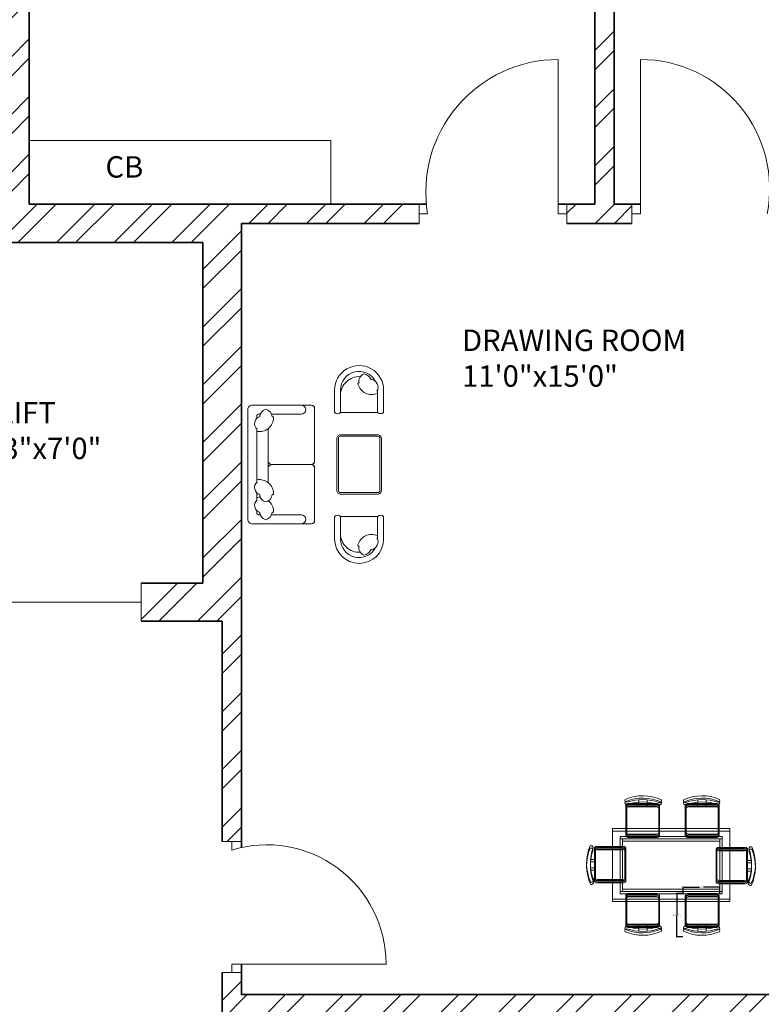
# Model space of a CAD drawing. Units: inches. Extents: x 2168 to 3056, y 1130 to 2629.
# Tile 33 of 42: x 2598 to 2771, y 2079 to 2308. Entities that reach past the tile are written whole.
import ezdxf

# ---------------------------------------------------------------- set-up
doc = ezdxf.new("R2010")
doc.units = ezdxf.units.IN
for name, color, linetype, lineweight in [('A-ANNO-DIMS', 2, 'Continuous', 18), ('A-ANNO-TEXT', 7, 'Continuous', 18), ('A-AREA-IDEN', 7, 'Continuous', 18), ('A-DOOR', 21, 'Continuous', 18), ('A-EQPM-ELEV', 7, 'Continuous', 18), ('A-FLOR-CASE', 71, 'Continuous', 18), ('A-FURN', 8, 'Continuous', 13), ('A-WALL', 7, 'Continuous', 35)]:
    doc.layers.add(name, color=color, linetype=linetype, lineweight=lineweight)
doc.layers.add('A-WALL-PATT', color=143, linetype='Continuous', lineweight=13, true_color=0x7aafdf)
doc.styles.get("Standard").update_dxf_attribs({"font": 'arial.ttf'})
doc.dimstyles.get("Standard").update_dxf_attribs({"dimtxt": 0.18, "dimasz": 0.18, "dimexe": 0.18, "dimexo": 0.0625, "dimgap": 0.09, "dimtad": 0, "dimtih": 1, "dimtoh": 1, "dimdec": 4, "dimzin": 0, "dimdsep": 46, "dimtxsty": 'Standard', "dimcen": 0.09, "dimadec": 0, "dimazin": 0, "dimtfac": 1, "dimtdec": 4, "dimtofl": 0, "dimtmove": 0, "dimatfit": 3, "dimfxl": 1, "dimtolj": 1, "dimtzin": 0, "dimarcsym": 0})

# ---------------------------------------------------------------- blocks, each defined once
blk = doc.blocks.new('A$C1352')
at = {"color": 0}
for points in [[(0.003, 0.053), (0.003, 0.553, -0.414214), (0.053, 0.603), (0.753, 0.603, -0.414214), (0.803, 0.553), (0.803, 0.053, -0.414214), (0.753, 0.003), (0.053, 0.003, -0.414214)], [(0.023, 0.053), (0.023, 0.553, -0.414214), (0.053, 0.583), (0.753, 0.583, -0.414214), (0.783, 0.553), (0.783, 0.053, -0.414214), (0.753, 0.023), (0.053, 0.023, -0.414214)]]:
    blk.add_lwpolyline(points, format="xyb", close=True, dxfattribs=at)
blk = doc.blocks.new('CHAIR-LOUNGE')
blk.add_line((10.04, 5.71), (10.04, 10.98))
at = {"ltscale": 0.03}
blk.add_lwpolyline([(10.04, 10.98, -0.369229), (11.42, 10.98), (11.42, 5.7, -1), (0, 5.72), (0, 10.99, -0.369229), (1.39, 10.99)], format="xyb", close=True, dxfattribs=at)
blk.add_lwpolyline([(9.55, 3.71, -0.785087), (1.38, 5.71), (1.39, 10.99)], format="xyb")
for centre, radius, start, end in [((5.71, 6.93), 4.33, 179.9461, 273.658), ((8.67, 3.43), 3.35, 67.0143, 164.2857), ((8.41, 5.02), 1.73, 272.9922, 34.1401), ((5.71, 5.71), 4.33, 358.8536, 359.9461), ((5.63, 4.23), 0.207, 150.6238, 293.7423), ((7.44, 3.63), 1.78, 166.6403, 249.4695), ((6.65, 3.91), 1.95, 274.9999, 341.3534)]:
    blk.add_arc(centre, radius, start, end)
blk = doc.blocks.new('TABLE-DINING')
for points in [[(0, 17.02), (27.45, 17.02), (27.45, 0.55), (0, 0.55)], [(0, 17.02), (27.45, 17.02), (27.45, 0.55), (0, 0.55)], [(0, 16.47), (27.45, 16.47), (27.45, 0), (0, 0)], [(0, 16.47), (27.45, 16.47), (27.45, 0), (0, 0)], [(1.83, 15.19), (25.62, 15.19), (25.62, 2.38), (1.83, 2.38)], [(1.83, 15.19), (25.62, 15.19), (25.62, 2.38), (1.83, 2.38)], [(1.83, 14.64), (25.62, 14.64), (25.62, 1.83), (1.83, 1.83)], [(1.83, 14.64), (25.62, 14.64), (25.62, 1.83), (1.83, 1.83)], [(2.38, 14.64), (25.07, 14.64), (25.07, 2.93), (2.38, 2.93)], [(2.38, 14.64), (25.07, 14.64), (25.07, 2.93), (2.38, 2.93)], [(2.38, 14.09), (25.07, 14.09), (25.07, 2.38), (2.38, 2.38)], [(2.38, 14.09), (25.07, 14.09), (25.07, 2.38), (2.38, 2.38)]]:
    blk.add_lwpolyline(points, close=True)
blk = doc.blocks.new('CUPBOARD-BEDROOM')
blk.add_lwpolyline([(0, 14.89), (70.36, 14.89), (70.36, 0), (0, 0)], close=True)
blk = doc.blocks.new('CHAIR-DINING-SIDE')
for points in [[(7.85, 2.38, 0.414214), (8.33, 2.86), (8.33, 9.24, 0.414214), (7.85, 9.73), (0.91, 9.73, 0.414214), (0.42, 9.24), (0.42, 2.86, 0.414214), (0.91, 2.38), (7.85, 2.38)], [(7.85, 2.38, 0.414214), (8.33, 2.86), (8.33, 9.24, 0.414214), (7.85, 9.73), (0.91, 9.73, 0.414214), (0.42, 9.24), (0.42, 2.86, 0.414214), (0.91, 2.38), (7.85, 2.38)], [(7.85, 1.83, 0.414214), (8.33, 2.31), (8.33, 8.69, 0.414214), (7.85, 9.18), (0.91, 9.18, 0.414214), (0.42, 8.69), (0.42, 2.31, 0.414214), (0.91, 1.83), (7.85, 1.83)], [(7.85, 1.83, 0.414214), (8.33, 2.31), (8.33, 8.69, 0.414214), (7.85, 9.18), (0.91, 9.18, 0.414214), (0.42, 8.69), (0.42, 2.31, 0.414214), (0.91, 1.83), (7.85, 1.83)], [(3.34, 2.38), (3.34, 1.5, -0.064759)], [(3.34, 2.38), (3.34, 1.5, -0.064759)], [(8.06, 2.08, -0.175809), (0.59, 2.13, 0.578392), (0.02, 1.51, 0.214524), (8.46, 1.4, 0.552014), (8.06, 2.08, -0.065079)], [(8.06, 2.08, -0.175809), (0.59, 2.13, 0.578392), (0.02, 1.51, 0.214524), (8.46, 1.4, 0.552014), (8.06, 2.08, -0.065079)], [(8.06, 1.53, -0.175809), (0.59, 1.58, 0.578392), (0.02, 0.96, 0.214524), (8.46, 0.85, 0.552014), (8.06, 1.53, -0.065079)], [(8.06, 1.53, -0.175809), (0.59, 1.58, 0.578392), (0.02, 0.96, 0.214524), (8.46, 0.85, 0.552014), (8.06, 1.53, -0.065079)], [(3.34, 1.83), (3.34, 0.95, -0.064759)], [(3.34, 1.83), (3.34, 0.95, -0.064759)]]:
    blk.add_lwpolyline(points, format="xyb")
for points in [[(7.84, 2.6), (1.13, 2.6, -0.414214), (0.64, 3.08), (0.64, 9.02, -0.414214), (1.13, 9.51), (7.84, 9.51, -0.512069), (8.11, 9.02), (8.11, 3.08, -0.512069)], [(7.84, 2.6), (1.13, 2.6, -0.414214), (0.64, 3.08), (0.64, 9.02, -0.414214), (1.13, 9.51), (7.84, 9.51, -0.512069), (8.11, 9.02), (8.11, 3.08, -0.512069)], [(7.84, 2.05), (1.13, 2.05, -0.414214), (0.64, 2.53), (0.64, 8.48, -0.414214), (1.13, 8.96), (7.84, 8.96, -0.512069), (8.11, 8.48), (8.11, 2.53, -0.512069)], [(7.84, 2.05), (1.13, 2.05, -0.414214), (0.64, 2.53), (0.64, 8.48, -0.414214), (1.13, 8.96), (7.84, 8.96, -0.512069), (8.11, 8.48), (8.11, 2.53, -0.512069)]]:
    blk.add_lwpolyline(points, format="xyb", close=True)
for points in [[(5.29, 1.48), (5.29, 2.38)], [(5.29, 1.48), (5.29, 2.38)], [(5.29, 0.93), (5.29, 1.83)], [(5.29, 0.93), (5.29, 1.83)]]:
    blk.add_lwpolyline(points)
blk = doc.blocks.new('*D26')
at = {"layer": 'A-ANNO-DIMS', "color": 0, "lineweight": -2, "transparency": 16777216}
for p, q in [((2752.83, 2104.47), (2751.21, 2104.47)), ((2751.39, 2104.29), (2751.39, 2099.63)), ((2751.39, 2094.6), (2751.39, 2099.26)), ((2752.83, 2094.42), (2751.21, 2094.42))]:
    blk.add_line(p, q, dxfattribs=at)
at = {"layer": 'A-ANNO-DIMS', "color": 0, "transparency": 16777216}
for points in [[(2751.36, 2104.29), (2751.42, 2104.29), (2751.39, 2104.47)], [(2751.36, 2094.6), (2751.42, 2094.6), (2751.39, 2094.42)]]:
    blk.add_solid(points, dxfattribs=at)
at = {"layer": 'Defpoints', "color": 0, "transparency": 16777216}
for p in [(2751.39, 2104.47), (2752.9, 2104.47), (2752.9, 2094.42)]:
    blk.add_point(p, dxfattribs=at)
at = {"layer": 'A-ANNO-DIMS', "color": 0, "transparency": 16777216, "insert": (2751.39, 2099.45), "char_height": 0.18, "attachment_point": 5}
blk.add_mtext('\\A1;SIDE CHAIR 10 TYP.', dxfattribs=at)
blk = doc.blocks.new('*D27')
at = {"layer": 'A-ANNO-DIMS', "color": 0, "lineweight": -2, "transparency": 16777216}
for p, q in [((2752.9, 2104.54), (2752.9, 2106.16)), ((2753.08, 2105.98), (2756.72, 2105.98)), ((2761.28, 2105.98), (2757.64, 2105.98)), ((2761.46, 2104.54), (2761.46, 2106.16))]:
    blk.add_line(p, q, dxfattribs=at)
at = {"layer": 'A-ANNO-DIMS', "color": 0, "transparency": 16777216}
for points in [[(2753.08, 2106.01), (2753.08, 2105.95), (2752.9, 2105.98)], [(2761.28, 2106.01), (2761.28, 2105.95), (2761.46, 2105.98)]]:
    blk.add_solid(points, dxfattribs=at)
at = {"layer": 'Defpoints', "color": 0, "transparency": 16777216}
for p in [(2761.46, 2105.98), (2752.9, 2104.47), (2761.46, 2104.47)]:
    blk.add_point(p, dxfattribs=at)
at = {"layer": 'A-ANNO-DIMS', "color": 0, "transparency": 16777216, "insert": (2757.18, 2105.98), "char_height": 0.18, "attachment_point": 5}
blk.add_mtext('\\A1;9 TYP.', dxfattribs=at)

msp = doc.modelspace()

# ---------------------------------------------------------------- hatches: boundary and pattern name
at = {"layer": 'A-WALL-PATT'}
h = msp.add_hatch(dxfattribs=at)
h.set_pattern_fill('ANSI32', color=256)
h.paths.add_polyline_path([(2463.8, 2409.39), (2467.39, 2409.39), (2467.39, 2413.89), (2454.77, 2413.89), (2454.77, 2411.64), (2454.77, 2409.39), (2459.3, 2409.39), (2459.3, 2265.39), (2455.64, 2265.39), (2455.64, 2260.89), (2467.35, 2260.89), (2467.35, 2263.14), (2467.35, 2265.39), (2463.8, 2265.39)])
h.paths.add_polyline_path([(2431.6, 2413.89), (2409.65, 2413.89), (2409.65, 2409.39), (2431.6, 2409.39), (2431.6, 2411.64)])
h.paths.add_polyline_path([(2349.65, 2413.89), (2331.8, 2413.89), (2331.8, 2362.67), (2336.3, 2362.67), (2336.3, 2409.39), (2349.65, 2409.39), (2349.65, 2411.64)])
h.paths.add_polyline_path([(2634.15, 2411.64), (2634.15, 2413.89), (2562.29, 2413.89), (2562.29, 2409.39), (2595.8, 2409.39), (2595.8, 2280.31), (2595.83, 2280.31), (2595.83, 2265.39), (2499.91, 2265.39), (2499.91, 2260.89), (2550.8, 2260.89), (2550.8, 2117.31), (2555.3, 2117.31), (2555.3, 2168.08), (2571.93, 2168.08), (2571.93, 2176.89), (2559.8, 2176.89), (2559.8, 2256.39), (2640.8, 2256.39), (2640.8, 2176.89), (2626.43, 2176.89), (2626.43, 2168.08), (2645.3, 2168.08), (2645.3, 2116.64), (2649.8, 2116.64), (2649.8, 2260.89), (2691.25, 2260.89), (2691.25, 2263.14), (2691.25, 2265.39), (2670.65, 2265.39), (2670.65, 2265.36), (2600.3, 2265.36), (2600.3, 2280.26), (2600.3, 2409.39), (2634.15, 2409.39)])
h.paths.add_polyline_path([(2600.3, 2473.89), (2612.84, 2473.89), (2612.84, 2478.39), (2572.64, 2478.39), (2572.64, 2473.89), (2595.8, 2473.89), (2595.8, 2413.89), (2600.3, 2413.89)])
h.paths.add_polyline_path([(2535.8, 2473.89), (2548.64, 2473.89), (2548.64, 2478.39), (2531.4, 2478.39), (2531.4, 2413.89), (2521.6, 2413.89), (2521.6, 2409.39), (2539.24, 2409.39), (2539.24, 2411.64), (2539.24, 2413.89), (2535.8, 2413.89)])
h.paths.add_polyline_path([(2664.8, 2478.39), (2636.84, 2478.39), (2636.84, 2473.89), (2660.3, 2473.89), (2660.3, 2413.89), (2656.17, 2413.89), (2656.17, 2409.39), (2671.68, 2409.39), (2671.68, 2411.64), (2671.68, 2413.89), (2664.8, 2413.89)])
h.paths.add_polyline_path([(2705.94, 2413.89), (2695.68, 2413.89), (2695.68, 2409.39), (2705.94, 2409.39)])
h.paths.add_polyline_path([(2741.35, 2413.89), (2728.73, 2413.89), (2728.73, 2411.64), (2728.73, 2409.39), (2732.3, 2409.39), (2732.3, 2265.39), (2725.73, 2265.39), (2725.73, 2260.89), (2740.92, 2260.89), (2740.92, 2263.14), (2740.92, 2265.39), (2736.8, 2265.39), (2736.8, 2409.39), (2741.35, 2409.39)])
h.paths.add_polyline_path([(2785.65, 2413.89), (2764.55, 2413.89), (2764.49, 2409.39), (2785.65, 2409.39), (2785.65, 2411.64)])
h.paths.add_polyline_path([(2864.3, 2413.89), (2845.65, 2413.89), (2845.65, 2409.39), (2859.8, 2409.39), (2859.8, 2368.43), (2864.3, 2368.43)])
h.paths.add_polyline_path([(2864.3, 2308.43), (2862.05, 2308.43), (2859.8, 2308.43), (2859.8, 2265.39), (2774.48, 2265.39), (2774.48, 2263.14), (2774.48, 2260.89), (2781.8, 2260.89), (2781.8, 2226.65), (2786.3, 2226.65), (2786.3, 2260.89), (2859.8, 2260.89), (2859.8, 2241.35), (2864.3, 2241.35)])
h.paths.add_polyline_path([(2864.3, 2217.35), (2862.05, 2217.35), (2859.8, 2217.35), (2859.8, 2200.89), (2786.3, 2200.89), (2786.3, 2205.93), (2784.05, 2205.93), (2781.8, 2205.93), (2781.8, 2150.97), (2786.3, 2150.97), (2786.3, 2161.89), (2859.8, 2161.89), (2859.8, 2144.42), (2864.3, 2144.42)])
h.paths.add_polyline_path([(2859.8, 2196.39), (2859.8, 2166.39), (2786.3, 2166.39), (2786.3, 2196.39)], flags=16)
h.paths.add_polyline_path([(2864.3, 2108.42), (2862.05, 2108.42), (2859.8, 2108.42), (2859.8, 2080.89), (2786.3, 2080.89), (2786.3, 2111.99), (2781.8, 2111.99), (2781.8, 2080.89), (2649.8, 2080.89), (2649.8, 2086.04), (2647.55, 2086.04), (2645.3, 2086.04), (2645.3, 2071.74), (2649.8, 2071.74), (2649.8, 2076.39), (2781.8, 2076.39), (2781.8, 2041.79), (2786.3, 2041.79), (2786.3, 2076.39), (2859.8, 2076.39), (2859.8, 2058.58), (2864.3, 2058.58)])
h.paths.add_polyline_path([(2864.3, 2022.58), (2859.8, 2022.58), (2859.8, 1992.39), (2786.3, 1992.39), (2786.3, 1999.57), (2781.8, 1999.57), (2781.8, 1848.09), (2784.05, 1848.09), (2786.3, 1848.09), (2786.3, 1851.39), (2859.8, 1851.39), (2859.8, 1838.26), (2864.3, 1838.26)], flags=17)
h.paths.add_polyline_path([(2859.8, 1987.89), (2859.8, 1855.89), (2786.3, 1855.89), (2786.3, 1987.89)], flags=16)
h.paths.add_polyline_path([(2823.05, 1987.89), (2841.42, 1921.89), (2823.05, 1855.89)], flags=0)
h.paths.add_polyline_path([(2864.3, 1814.26), (2859.8, 1814.26), (2859.8, 1791.39), (2786.3, 1791.39), (2786.3, 1825.66), (2784.05, 1825.66), (2781.8, 1825.66), (2781.8, 1791.39), (2720.15, 1791.39), (2720.15, 1791.27), (2649.8, 1791.27), (2649.8, 1806.16), (2649.8, 2038.98), (2647.55, 2038.98), (2645.3, 2038.98), (2645.3, 1783.93), (2649.8, 1783.93), (2649.8, 1786.89), (2781.8, 1786.89), (2781.8, 1746.79), (2786.3, 1746.79), (2786.3, 1786.89), (2859.8, 1786.89), (2859.8, 1770.08), (2864.3, 1770.08)])
h.paths.add_polyline_path([(2864.3, 1734.08), (2862.05, 1734.08), (2859.8, 1734.08), (2859.8, 1705.89), (2786.3, 1705.89), (2786.3, 1714.17), (2781.8, 1714.17), (2781.8, 1660.53), (2786.3, 1660.53), (2786.3, 1666.89), (2859.8, 1666.89), (2859.8, 1648.34), (2864.3, 1648.34)])
h.paths.add_polyline_path([(2786.3, 1701.39), (2859.8, 1701.39), (2859.8, 1671.39), (2786.3, 1671.39)], flags=16)
h.paths.add_polyline_path([(2649.8, 1756.58), (2647.55, 1756.58), (2645.3, 1756.58), (2645.3, 1606.89), (2555.3, 1606.89), (2555.3, 1749.51), (2553.05, 1749.51), (2550.8, 1749.51), (2550.8, 1606.89), (2503.01, 1606.89), (2503.01, 1604.64), (2503.01, 1602.39), (2595.8, 1602.39), (2595.85, 1602.39), (2595.85, 1587.5), (2595.8, 1458.39), (2561.5, 1458.39), (2561.5, 1456.14), (2561.5, 1453.89), (2595.8, 1453.89), (2595.8, 1381.89), (2573.44, 1381.89), (2573.44, 1377.39), (2613.01, 1377.39), (2613.01, 1379.64), (2613.01, 1381.89), (2600.3, 1381.89), (2600.3, 1453.89), (2634.33, 1453.89), (2634.33, 1458.39), (2600.3, 1458.39), (2600.3, 1602.39), (2670.65, 1602.39), (2694.09, 1602.39), (2694.09, 1606.89), (2649.8, 1606.89)])
h.paths.add_polyline_path([(2736.8, 1602.39), (2741.56, 1602.39), (2741.56, 1606.89), (2726.2, 1606.89), (2726.2, 1604.64), (2726.2, 1602.39), (2732.3, 1602.39), (2732.3, 1458.39), (2727.9, 1458.39), (2727.9, 1453.89), (2740.82, 1453.89), (2740.82, 1456.14), (2740.82, 1458.39), (2736.8, 1458.39)])
h.paths.add_polyline_path([(2859.8, 1606.89), (2786.3, 1606.89), (2786.3, 1637.33), (2784.05, 1637.33), (2781.8, 1637.33), (2781.8, 1606.89), (2775.61, 1606.89), (2775.61, 1602.39), (2859.8, 1602.39)])
h.paths.add_polyline_path([(2864.3, 1624.34), (2862.05, 1624.34), (2859.8, 1624.34), (2859.8, 1570.39), (2864.3, 1570.39)])
h.paths.add_polyline_path([(2864.3, 1510.39), (2862.05, 1510.39), (2859.8, 1510.39), (2859.8, 1458.39), (2846.73, 1458.39), (2846.73, 1456.14), (2846.73, 1453.89), (2864.3, 1453.89)])
h.paths.add_polyline_path([(2786.73, 1458.39), (2765.44, 1458.39), (2765.44, 1453.89), (2786.73, 1453.89)])
h.paths.add_polyline_path([(2706, 1458.39), (2695.36, 1458.39), (2695.36, 1453.89), (2706, 1453.89), (2706, 1456.14)])
h.paths.add_polyline_path([(2671.36, 1456.14), (2671.36, 1458.39), (2655.99, 1458.39), (2655.99, 1456.14), (2655.99, 1453.89), (2660.3, 1453.89), (2660.3, 1381.89), (2637.01, 1381.89), (2637.01, 1377.39), (2664.8, 1377.39), (2664.8, 1453.89), (2671.36, 1453.89)], flags=17)
h.paths.add_polyline_path([(2539.83, 1458.39), (2520.24, 1458.39), (2520.24, 1453.89), (2531.3, 1453.89), (2531.3, 1377.39), (2546.45, 1377.39), (2546.45, 1379.64), (2546.45, 1381.89), (2535.8, 1381.89), (2535.8, 1453.89), (2539.83, 1453.89)], flags=17)
h.paths.add_polyline_path([(2496.24, 1458.39), (2489.13, 1458.39), (2489.13, 1453.89), (2496.24, 1453.89), (2496.24, 1456.14)])
h.paths.add_polyline_path([(2467.43, 1456.14), (2467.43, 1458.39), (2463.8, 1458.39), (2463.8, 1602.39), (2468.24, 1602.39), (2468.24, 1605.7), (2468.24, 1606.89), (2454.6, 1606.89), (2454.6, 1602.39), (2459.3, 1602.39), (2459.3, 1458.39), (2454.24, 1458.39), (2454.24, 1453.89), (2467.43, 1453.89)])
h.paths.add_polyline_path([(2431.6, 1456.14), (2431.6, 1458.39), (2411.39, 1458.39), (2411.39, 1453.89), (2431.6, 1453.89)])
h.paths.add_polyline_path([(2351.39, 1458.39), (2336.3, 1458.39), (2336.3, 1490.69), (2334.05, 1490.69), (2331.8, 1490.69), (2331.8, 1453.89), (2351.39, 1453.89), (2351.39, 1456.14)])
h.paths.add_polyline_path([(2336.3, 1629.7), (2331.8, 1629.7), (2331.8, 1552.32), (2336.3, 1552.32), (2336.3, 1602.39), (2406.65, 1602.39), (2423.47, 1602.39), (2423.47, 1606.89), (2418.8, 1606.89), (2418.8, 1643.68), (2416.55, 1643.68), (2414.3, 1643.68), (2414.3, 1606.89), (2336.3, 1606.89)])
h.paths.add_polyline_path([(2418.8, 1714.38), (2414.3, 1714.38), (2414.3, 1705.89), (2336.3, 1705.89), (2336.3, 1731.32), (2334.05, 1731.32), (2331.8, 1731.32), (2331.8, 1653.7), (2334.05, 1653.7), (2336.3, 1653.7), (2336.3, 1666.89), (2414.3, 1666.89), (2414.3, 1663.59), (2418.8, 1663.59)])
h.paths.add_polyline_path([(2336.3, 1701.39), (2414.3, 1701.39), (2414.3, 1671.39), (2336.3, 1671.39)], flags=16)
h.paths.add_polyline_path([(2555.3, 2040.06), (2550.8, 2040.06), (2550.8, 1791.39), (2550.56, 1791.2), (2480.2, 1791.2), (2418.8, 1791.39), (2418.8, 1825.45), (2416.55, 1825.45), (2414.3, 1825.45), (2414.3, 1791.39), (2336.3, 1791.39), (2336.3, 1806.41), (2331.8, 1806.41), (2331.8, 1767.32), (2336.3, 1767.32), (2336.3, 1786.89), (2414.3, 1786.89), (2414.3, 1745.46), (2418.8, 1745.46), (2418.8, 1786.89), (2550.8, 1786.89), (2550.8, 1783.01), (2555.3, 1783.01)])
h.paths.add_polyline_path([(2418.8, 1923.39), (2423.21, 1923.39), (2423.21, 1925.64), (2423.21, 1927.89), (2418.8, 1927.89), (2418.8, 2000.05), (2414.3, 2000.05), (2414.3, 1992.39), (2336.3, 1992.39), (2336.3, 1987.89), (2414.3, 1987.89), (2414.3, 1855.89), (2336.3, 1855.89), (2336.3, 1851.39), (2414.3, 1851.39), (2414.3, 1846.76), (2418.8, 1846.76)], flags=17)
h.paths.add_polyline_path([(2336.3, 2019.29), (2334.05, 2019.29), (2331.8, 2019.29), (2331.8, 1830.41), (2336.3, 1830.41)], flags=17)
h.paths.add_polyline_path([(2550.8, 1927.89), (2453.54, 1927.89), (2453.54, 1925.64), (2453.54, 1923.39), (2550.8, 1923.39)], flags=17)
h.paths.add_polyline_path([(2744.99, 1927.89), (2649.8, 1927.89), (2649.8, 1923.39), (2744.99, 1923.39), (2744.99, 1925.64)], flags=17)
h.paths.add_polyline_path([(2555.3, 2086.46), (2553.05, 2086.46), (2550.8, 2086.46), (2550.8, 2080.89), (2418.8, 2080.89), (2336.3, 2080.89), (2336.3, 2115.4), (2334.05, 2115.4), (2331.8, 2115.4), (2331.8, 2055.29), (2336.3, 2055.29), (2336.3, 2076.39), (2550.8, 2076.39), (2550.8, 2071.54), (2555.3, 2071.54)])
h.paths.add_polyline_path([(2418.8, 2121.39), (2414.3, 2121.39), (2414.3, 2080.89), (2418.8, 2080.89)])
h.paths.add_polyline_path([(2418.8, 2076.39), (2414.3, 2076.39), (2414.3, 2035.12), (2418.8, 2035.12)])
h.paths.add_polyline_path([(2422.87, 2263.14), (2422.87, 2265.39), (2406.65, 2265.39), (2406.65, 2265.36), (2336.3, 2265.36), (2336.3, 2280.25), (2336.3, 2302.67), (2334.05, 2302.67), (2331.8, 2302.67), (2331.8, 2246.85), (2336.3, 2246.85), (2336.3, 2260.89), (2414.3, 2260.89), (2414.3, 2224), (2418.8, 2224), (2418.8, 2260.89), (2422.87, 2260.89)])
h.paths.add_polyline_path([(2418.8, 2204.78), (2416.55, 2204.78), (2414.3, 2204.78), (2414.3, 2200.89), (2336.3, 2200.89), (2336.3, 2220.85), (2331.8, 2220.85), (2331.8, 2151.4), (2336.3, 2151.4), (2336.3, 2161.89), (2414.3, 2161.89), (2414.3, 2153.73), (2418.8, 2153.73)])
h.paths.add_polyline_path([(2414.3, 2196.39), (2414.3, 2166.39), (2336.3, 2166.39), (2336.3, 2196.39)], flags=16)
h.paths.add_polyline_path([(2375.3, 2181.39), (2336.3, 2166.39), (2336.3, 2196.39)], flags=0)
h.paths.add_polyline_path([(2809.6, 2172.34), (2838.8, 2172.34), (2838.8, 2191), (2809.6, 2191)], flags=8)
h.paths.add_polyline_path([(2849.75, 1919.59), (2849.75, 1952.67), (2831.09, 1952.67), (2831.09, 1919.59)], flags=8)
h.paths.add_polyline_path([(2808.87, 1901.97), (2808.87, 1937.85), (2790.15, 1937.85), (2790.15, 1901.97)], flags=8)
h.paths.add_polyline_path([(2806.28, 1671.9), (2835.49, 1671.9), (2835.49, 1690.55), (2806.28, 1690.55)], flags=8)
h.paths.add_polyline_path([(2353.19, 1676.55), (2382.39, 1676.55), (2382.39, 1695.21), (2353.19, 1695.21)], flags=8)
h.paths.add_polyline_path([(2360.08, 1832.31), (2389.24, 1832.31), (2389.24, 1850.97), (2360.08, 1850.97)], flags=25)
h.paths.add_polyline_path([(2354.82, 2167.82), (2384.03, 2167.82), (2384.03, 2186.48), (2354.82, 2186.48)], flags=8)

# ---------------------------------------------------------------- linework, layer by layer
at = {"layer": 'A-DOOR'}
for p, q in [((2723.73, 2263.14), (2723.73, 2299.14)), ((2742.92, 2263.14), (2742.92, 2299.14)), ((2691.25, 2265.39), (2691.25, 2260.89)), ((2725.73, 2265.39), (2725.73, 2260.89)), ((2740.92, 2265.39), (2740.92, 2260.89)), ((2691.25, 2260.89), (2691.25, 2263.14)), ((2691.25, 2263.14), (2693.25, 2263.14)), ((2725.73, 2263.14), (2723.73, 2263.14)), ((2725.73, 2260.89), (2725.73, 2263.14)), ((2740.92, 2260.89), (2740.92, 2263.14)), ((2740.92, 2263.14), (2742.92, 2263.14)), ((2645.3, 2116.64), (2649.8, 2116.64)), ((2649.8, 2116.64), (2647.55, 2116.64)), ((2647.55, 2116.64), (2647.55, 2114.64)), ((2647.55, 2086.04), (2647.55, 2088.04)), ((2647.55, 2088.04), (2683.55, 2088.04)), ((2645.3, 2086.04), (2649.8, 2086.04)), ((2649.8, 2086.04), (2647.55, 2086.04))]:
    msp.add_line(p, q, dxfattribs=at)
for centre, radius, start, end in [((2723.73, 2268.23), 30.9, 90, 189.4908), ((2742.92, 2269), 30.14, 348.7897, 90), ((2655.72, 2088.04), 27.83, 360, 107.0763)]:
    msp.add_arc(centre, radius, start, end, dxfattribs=at)
at = {"layer": 'A-EQPM-ELEV'}
for p, q in [((2626.43, 2176.89), (2626.43, 2168.08)), ((2626.43, 2172.48), (2571.93, 2172.48))]:
    msp.add_line(p, q, dxfattribs=at)
at = {"layer": 'A-FURN'}
for p, q in [((2653.38, 2216.04), (2653.38, 2215.4)), ((2654.21, 2216.38), (2653.73, 2216.38)), ((2663.76, 2216.38), (2656.84, 2216.38)), ((2653.38, 2212.9), (2653.38, 2200.49)), ((2653.38, 2197.35), (2653.38, 2197.99)), ((2653.38, 2197.99), (2653.38, 2196.33)), ((2653.38, 2193.2), (2653.38, 2193.84)), ((2654.21, 2192.85), (2653.73, 2192.85)), ((2656.84, 2192.85), (2663.76, 2192.85))]:
    msp.add_line(p, q, dxfattribs=at)
at = {"layer": 'A-FURN', "ltscale": 0.03}
msp.add_lwpolyline([(2666.19, 2204.63, 0.414214), (2666.88, 2205.32), (2666.88, 2217.77, 0.414214), (2666.19, 2218.46), (2652.34, 2218.46, 0.414214), (2651.31, 2217.42), (2651.31, 2191.81, 0.414214), (2652.34, 2190.78), (2666.19, 2190.78, 0.414214), (2666.88, 2191.47), (2666.88, 2203.92, 0.414214), (2666.19, 2204.61)], format="xyb", dxfattribs=at)
at = {"layer": 'A-FURN'}
for points in [[(2656.06, 2212.45), (2656.06, 2205.48, 0.414214), (2656.93, 2204.62), (2666.01, 2204.62, 0.414214), (2666.88, 2205.48), (2666.88, 2217.6, 0.414214), (2666.01, 2218.46)], [(2656.06, 2200.35), (2656.06, 2203.75, -0.414214), (2656.93, 2204.62), (2666.01, 2204.62, -0.414214), (2666.88, 2203.75), (2666.88, 2191.64, -0.414214), (2666.01, 2190.78)], [(2739.75, 2125.79, -0.175809), (2747.22, 2125.73, 0.578392), (2747.79, 2126.35, 0.214524), (2739.35, 2126.47, 0.552014), (2739.75, 2125.79, -0.065079)], [(2739.75, 2125.79, -0.175809), (2747.22, 2125.73, 0.578392), (2747.79, 2126.35, 0.214524), (2739.35, 2126.47, 0.552014), (2739.75, 2125.79, -0.065079)], [(2739.75, 2125.24, -0.175809), (2747.22, 2125.18, 0.578392), (2747.79, 2125.8, 0.214524), (2739.35, 2125.92, 0.552014), (2739.75, 2125.24, -0.065079)], [(2739.75, 2125.24, -0.175809), (2747.22, 2125.18, 0.578392), (2747.79, 2125.8, 0.214524), (2739.35, 2125.92, 0.552014), (2739.75, 2125.24, -0.065079)], [(2744.47, 2125.49), (2744.47, 2126.36, -0.064759)], [(2744.47, 2125.49), (2744.47, 2126.36, -0.064759)], [(2744.47, 2124.94), (2744.47, 2125.82, -0.064759)], [(2744.47, 2124.94), (2744.47, 2125.82, -0.064759)], [(2746.91, 2125.49), (2739.97, 2125.49, 0.414214), (2739.48, 2125), (2739.48, 2118.62, 0.414214), (2739.97, 2118.13), (2746.91, 2118.13, 0.414214), (2747.39, 2118.62), (2747.39, 2125, 0.414214), (2746.91, 2125.49)], [(2746.91, 2125.49), (2739.97, 2125.49, 0.414214), (2739.48, 2125), (2739.48, 2118.62, 0.414214), (2739.97, 2118.13), (2746.91, 2118.13, 0.414214), (2747.39, 2118.62), (2747.39, 2125, 0.414214), (2746.91, 2125.49)], [(2746.91, 2124.94), (2739.97, 2124.94, 0.414214), (2739.48, 2124.45), (2739.48, 2118.07, 0.414214), (2739.97, 2117.59), (2746.91, 2117.59, 0.414214), (2747.39, 2118.07), (2747.39, 2124.45, 0.414214), (2746.91, 2124.94)], [(2746.91, 2124.94), (2739.97, 2124.94, 0.414214), (2739.48, 2124.45), (2739.48, 2118.07, 0.414214), (2739.97, 2117.59), (2746.91, 2117.59, 0.414214), (2747.39, 2118.07), (2747.39, 2124.45, 0.414214), (2746.91, 2124.94)], [(2731.93, 2107.73, -0.578392), (2731.3, 2107.17, -0.214524), (2731.19, 2115.61, -0.552014), (2731.87, 2115.21, 0.175809), (2731.93, 2107.73)], [(2731.93, 2107.73, -0.578392), (2731.3, 2107.17, -0.214524), (2731.19, 2115.61, -0.552014), (2731.87, 2115.21, 0.175809), (2731.93, 2107.73)], [(2731.93, 2107.19, -0.578392), (2731.3, 2106.62, -0.214524), (2731.19, 2115.06, -0.552014), (2731.87, 2114.66, 0.175809), (2731.93, 2107.19)], [(2731.93, 2107.19, -0.578392), (2731.3, 2106.62, -0.214524), (2731.19, 2115.06, -0.552014), (2731.87, 2114.66, 0.175809), (2731.93, 2107.19)], [(2732.17, 2114.99, -0.414214), (2732.66, 2115.48), (2739.04, 2115.48, -0.414214), (2739.52, 2114.99), (2739.52, 2108.05, -0.414214), (2739.04, 2107.57), (2732.66, 2107.57, -0.414214), (2732.17, 2108.05), (2732.17, 2114.99)], [(2732.17, 2114.99, -0.414214), (2732.66, 2115.48), (2739.04, 2115.48, -0.414214), (2739.52, 2114.99), (2739.52, 2108.05, -0.414214), (2739.04, 2107.57), (2732.66, 2107.57, -0.414214), (2732.17, 2108.05), (2732.17, 2114.99)], [(2732.17, 2114.44, -0.414214), (2732.66, 2114.93), (2739.04, 2114.93, -0.414214), (2739.52, 2114.44), (2739.52, 2107.5, -0.414214), (2739.04, 2107.02), (2732.66, 2107.02, -0.414214), (2732.17, 2107.5), (2732.17, 2114.44)], [(2732.17, 2114.44, -0.414214), (2732.66, 2114.93), (2739.04, 2114.93, -0.414214), (2739.52, 2114.44), (2739.52, 2107.5, -0.414214), (2739.04, 2107.02), (2732.66, 2107.02, -0.414214), (2732.17, 2107.5), (2732.17, 2114.44)], [(2767.91, 2114.75, 0.414214), (2767.42, 2115.24), (2761.04, 2115.24, 0.414214), (2760.56, 2114.75), (2760.56, 2107.81, 0.414214), (2761.04, 2107.33), (2767.42, 2107.33, 0.414214), (2767.91, 2107.81), (2767.91, 2114.75)], [(2767.91, 2114.75, 0.414214), (2767.42, 2115.24), (2761.04, 2115.24, 0.414214), (2760.56, 2114.75), (2760.56, 2107.81, 0.414214), (2761.04, 2107.33), (2767.42, 2107.33, 0.414214), (2767.91, 2107.81), (2767.91, 2114.75)], [(2767.91, 2114.21, 0.414214), (2767.42, 2114.69), (2761.04, 2114.69, 0.414214), (2760.56, 2114.21), (2760.56, 2107.27, 0.414214), (2761.04, 2106.78), (2767.42, 2106.78, 0.414214), (2767.91, 2107.27), (2767.91, 2114.21)], [(2767.91, 2114.2, 0.414214), (2767.42, 2114.69), (2761.04, 2114.69, 0.414214), (2760.56, 2114.2), (2760.56, 2107.26, 0.414214), (2761.04, 2106.78), (2767.42, 2106.78, 0.414214), (2767.91, 2107.26), (2767.91, 2114.2)], [(2768.21, 2114.97, -0.175809), (2768.15, 2107.5, 0.578392), (2768.77, 2106.93, 0.214524), (2768.89, 2115.37, 0.552014), (2768.21, 2114.97, -0.065079)], [(2768.21, 2114.97, -0.175809), (2768.15, 2107.5, 0.578392), (2768.77, 2106.93, 0.214524), (2768.89, 2115.37, 0.552014), (2768.21, 2114.97, -0.065079)], [(2768.21, 2114.42, -0.175809), (2768.15, 2106.95, 0.578392), (2768.77, 2106.38, 0.214524), (2768.89, 2114.82, 0.552014), (2768.21, 2114.42, -0.065079)], [(2768.21, 2114.42, -0.175809), (2768.15, 2106.95, 0.578392), (2768.77, 2106.38, 0.214524), (2768.89, 2114.82, 0.552014), (2768.21, 2114.42, -0.065079)], [(2732.17, 2110.49), (2731.29, 2110.49, 0.064759)], [(2732.17, 2110.49), (2731.29, 2110.49, 0.064759)], [(2732.17, 2109.94), (2731.29, 2109.94, 0.064759)], [(2732.17, 2109.94), (2731.29, 2109.94, 0.064759)], [(2767.91, 2110.25), (2768.79, 2110.25, -0.064759)], [(2767.91, 2110.25), (2768.79, 2110.25, -0.064759)], [(2767.91, 2109.7), (2768.79, 2109.7, -0.064759)], [(2767.91, 2109.7), (2768.79, 2109.7, -0.064759)]]:
    msp.add_lwpolyline(points, format="xyb", dxfattribs=at)
for points in [[(2656.06, 2200.35), (2656.06, 2213.04)], [(2742.53, 2126.38), (2742.53, 2125.49)], [(2742.53, 2126.38), (2742.53, 2125.49)], [(2742.53, 2125.83), (2742.53, 2124.94)], [(2742.53, 2125.83), (2742.53, 2124.94)], [(2731.28, 2112.43), (2732.17, 2112.43)], [(2731.28, 2112.43), (2732.17, 2112.43)], [(2731.28, 2111.88), (2732.17, 2111.88)], [(2731.28, 2111.88), (2732.17, 2111.88)], [(2768.8, 2112.19), (2767.91, 2112.19)], [(2768.8, 2112.19), (2767.91, 2112.19)], [(2768.8, 2111.65), (2767.91, 2111.65)], [(2768.8, 2111.65), (2767.91, 2111.65)]]:
    msp.add_lwpolyline(points, dxfattribs=at)
for points in [[(2739.97, 2125.27), (2746.69, 2125.27, -0.414214), (2747.17, 2124.78), (2747.17, 2118.84, -0.414214), (2746.69, 2118.35), (2739.97, 2118.35, -0.512069), (2739.7, 2118.84), (2739.7, 2124.78, -0.512069)], [(2739.97, 2125.27), (2746.69, 2125.27, -0.414214), (2747.17, 2124.78), (2747.17, 2118.84, -0.414214), (2746.69, 2118.35), (2739.97, 2118.35, -0.512069), (2739.7, 2118.84), (2739.7, 2124.78, -0.512069)], [(2739.97, 2124.72), (2746.69, 2124.72, -0.414214), (2747.17, 2124.23), (2747.17, 2118.29, -0.414214), (2746.69, 2117.8), (2739.97, 2117.8, -0.512069), (2739.7, 2118.29), (2739.7, 2124.23, -0.512069)], [(2739.97, 2124.72), (2746.69, 2124.72, -0.414214), (2747.17, 2124.23), (2747.17, 2118.29, -0.414214), (2746.69, 2117.8), (2739.97, 2117.8, -0.512069), (2739.7, 2118.29), (2739.7, 2124.23, -0.512069)], [(2732.39, 2114.99), (2732.39, 2108.27, 0.414214), (2732.87, 2107.79), (2738.82, 2107.79, 0.414214), (2739.3, 2108.27), (2739.3, 2114.99, 0.512069), (2738.82, 2115.26), (2732.87, 2115.26, 0.512069)], [(2732.39, 2114.99), (2732.39, 2108.27, 0.414214), (2732.87, 2107.78), (2738.82, 2107.78, 0.414214), (2739.3, 2108.27), (2739.3, 2114.99, 0.512069), (2738.82, 2115.26), (2732.87, 2115.26, 0.512069)], [(2732.39, 2114.44), (2732.39, 2107.72, 0.414214), (2732.87, 2107.24), (2738.82, 2107.24, 0.414214), (2739.3, 2107.72), (2739.3, 2114.44, 0.512069), (2738.82, 2114.71), (2732.87, 2114.71, 0.512069)], [(2732.39, 2114.44), (2732.39, 2107.72, 0.414214), (2732.87, 2107.24), (2738.82, 2107.24, 0.414214), (2739.3, 2107.72), (2739.3, 2114.44, 0.512069), (2738.82, 2114.71), (2732.87, 2114.71, 0.512069)], [(2767.69, 2114.75), (2767.69, 2108.03, -0.414214), (2767.2, 2107.55), (2761.26, 2107.55, -0.414214), (2760.77, 2108.03), (2760.77, 2114.75, -0.512069), (2761.26, 2115.02), (2767.2, 2115.02, -0.512069)], [(2767.69, 2114.75), (2767.69, 2108.03, -0.414214), (2767.2, 2107.55), (2761.26, 2107.55, -0.414214), (2760.77, 2108.03), (2760.77, 2114.75, -0.512069), (2761.26, 2115.02), (2767.2, 2115.02, -0.512069)], [(2767.69, 2114.2), (2767.69, 2107.48, -0.414214), (2767.2, 2107), (2761.26, 2107, -0.414214), (2760.77, 2107.48), (2760.77, 2114.2, -0.512069), (2761.26, 2114.47), (2767.2, 2114.47, -0.512069)], [(2767.69, 2114.2), (2767.69, 2107.48, -0.414214), (2767.2, 2107), (2761.26, 2107, -0.414214), (2760.77, 2107.48), (2760.77, 2114.2, -0.512069), (2761.26, 2114.47), (2767.2, 2114.47, -0.512069)]]:
    msp.add_lwpolyline(points, format="xyb", close=True, dxfattribs=at)
for centre, radius, start, end in [((2656.02, 2215.65), 1.95, 109.1026, 175.4561), ((2655.18, 2215.73), 1.78, 0.743, 83.5721), ((2663.76, 2217.42), 1.04, 0, 90), ((2654.59, 2214.15), 1.73, 107.0949, 228.2428), ((2653.73, 2216.04), 0.346, 90, 180), ((2653.94, 2215.63), 3.35, 261.117, 358.3884), ((2657.09, 2215.59), 0.207, 344.7265, 127.845), ((2663.76, 2217.42), 1.04, 270, 0), ((2654.59, 2199.24), 1.73, 131.7572, 252.9051), ((2653.94, 2197.76), 3.35, 1.6116, 98.883), ((2653.94, 2193.61), 3.35, 84.881, 98.883), ((2656.02, 2197.74), 1.95, 184.5439, 250.8974), ((2655.18, 2197.66), 1.78, 276.4279, 359.257), ((2657.09, 2197.8), 0.207, 232.155, 15.2735), ((2654.59, 2195.08), 1.73, 131.7572, 252.9051), ((2653.94, 2193.61), 3.35, 1.6116, 49.376), ((2653.73, 2193.2), 0.346, 180, 270), ((2653.73, 2193.2), 0.346, 180, 270), ((2656.02, 2193.58), 1.95, 184.5439, 250.8974), ((2655.18, 2193.5), 1.78, 276.4279, 359.257), ((2657.09, 2193.65), 0.207, 232.155, 15.2735), ((2663.76, 2191.81), 1.04, 0, 90), ((2663.76, 2191.81), 1.04, 270, 0)]:
    msp.add_arc(centre, radius, start, end, dxfattribs=at)
at = {"layer": 'A-WALL'}
for p, q in [((2600.3, 2409.39), (2600.3, 2265.39)), ((2732.3, 2409.39), (2732.3, 2265.39)), ((2736.8, 2409.39), (2736.8, 2265.39)), ((2600.3, 2265.39), (2692.96, 2265.39)), ((2723.73, 2265.39), (2732.3, 2265.39)), ((2736.8, 2265.39), (2742.92, 2265.39)), ((2649.8, 2260.89), (2691.25, 2260.89)), ((2649.8, 2115.23), (2649.8, 2260.89)), ((2725.73, 2260.89), (2740.92, 2260.89)), ((2559.8, 2256.39), (2640.8, 2256.39)), ((2640.8, 2256.39), (2640.8, 2176.89)), ((2640.8, 2176.89), (2626.43, 2176.89)), ((2626.43, 2168.08), (2645.3, 2168.08)), ((2645.3, 2168.08), (2645.3, 2116.64)), ((2649.8, 2080.89), (2649.8, 2088.04)), ((2645.3, 2086.04), (2645.3, 2071.74)), ((2781.8, 2080.89), (2649.8, 2080.89)), ((2649.8, 2080.89), (2781.8, 2080.89))]:
    msp.add_line(p, q, dxfattribs=at)

# ---------------------------------------------------------------- block references
at = {"layer": 'A-FLOR-CASE'}
msp.add_blockref('CUPBOARD-BEDROOM', (2600.3, 2265.36), dxfattribs=at)
at = {"layer": 'A-FURN', "extrusion": (0, 0, -1), "zscale": -1, "rotation": 180}
for name, p in [('CHAIR-LOUNGE', (-2671.55, 2227.72)), ('CHAIR-DINING-SIDE', (-2752.93, 2127.31))]:
    msp.add_blockref(name, p, dxfattribs=at)
at = {"layer": 'A-FURN', "ltscale": 0.03, "xscale": 17.30251319894821, "yscale": 17.30251319894821, "zscale": 17.30251319894821, "rotation": 90}
msp.add_blockref('A$C1352', (2682.5, 2197.65), dxfattribs=at)
at = {"layer": 'A-FURN'}
for name, p in [('CHAIR-LOUNGE', (2671.55, 2181.52)), ('TABLE-DINING', (2736.35, 2102.61)), ('CHAIR-DINING-SIDE', (2752.93, 2094.74))]:
    msp.add_blockref(name, p, dxfattribs=at)
at = {"layer": 'A-FURN', "extrusion": (0, 0, -1), "zscale": -1}
msp.add_blockref('CHAIR-DINING-SIDE', (-2747.81, 2094.74), dxfattribs=at)

# ---------------------------------------------------------------- texts
at = {"layer": 'A-ANNO-TEXT', "insert": (2618.07, 2276.57), "char_height": 5, "attachment_point": 1}
msp.add_mtext_dynamic_manual_height_columns('CB', width=82.5793, gutter_width=12.5, heights=[0], dxfattribs=at)
at = {"layer": 'A-AREA-IDEN', "char_height": 5, "attachment_point": 1}
for s, width, insert in [('DRAWING ROOM\\P11\'0"x15\'0"', 85.0133, (2701.28, 2236.1)), ('            LIFT\\P\\pxt1;         6\'3"x7\'0"     ', 111.1942, (2574.59, 2219.2))]:
    msp.add_mtext_dynamic_manual_height_columns(s, width=width, gutter_width=12.5, heights=[0], dxfattribs=dict(at, insert=insert))

# ---------------------------------------------------------------- dimensions: what is measured, and where the dimension line sits
at = {"layer": 'A-ANNO-DIMS'}
dim = msp.add_linear_dim(base=(2761.46, 2105.98), p1=(2752.9, 2104.47), p2=(2761.46, 2104.47), text='<> TYP.', dimstyle='Standard', override={"dimdec": 0, "dimlfac": 1, "dimrnd": 0, "dimzin": 0, "dimdsep": 46, "dimlunit": 2}, dxfattribs=at)
dim.commit()
dim.dimension.update_dxf_attribs({"geometry": '*D27', "text_midpoint": (2757.18, 2105.98)})
dim = msp.add_linear_dim(base=(2751.39, 2104.47), p1=(2752.9, 2094.42), p2=(2752.9, 2104.47), angle=90, text='SIDE CHAIR <> TYP.', dimstyle='Standard', override={"dimdec": 0, "dimlfac": 1, "dimrnd": 0, "dimzin": 0, "dimdsep": 46, "dimlunit": 2}, dxfattribs=at)
dim.commit()
dim.dimension.update_dxf_attribs({"geometry": '*D26', "text_midpoint": (2751.39, 2099.45)})

doc.saveas('drawing.dxf')
